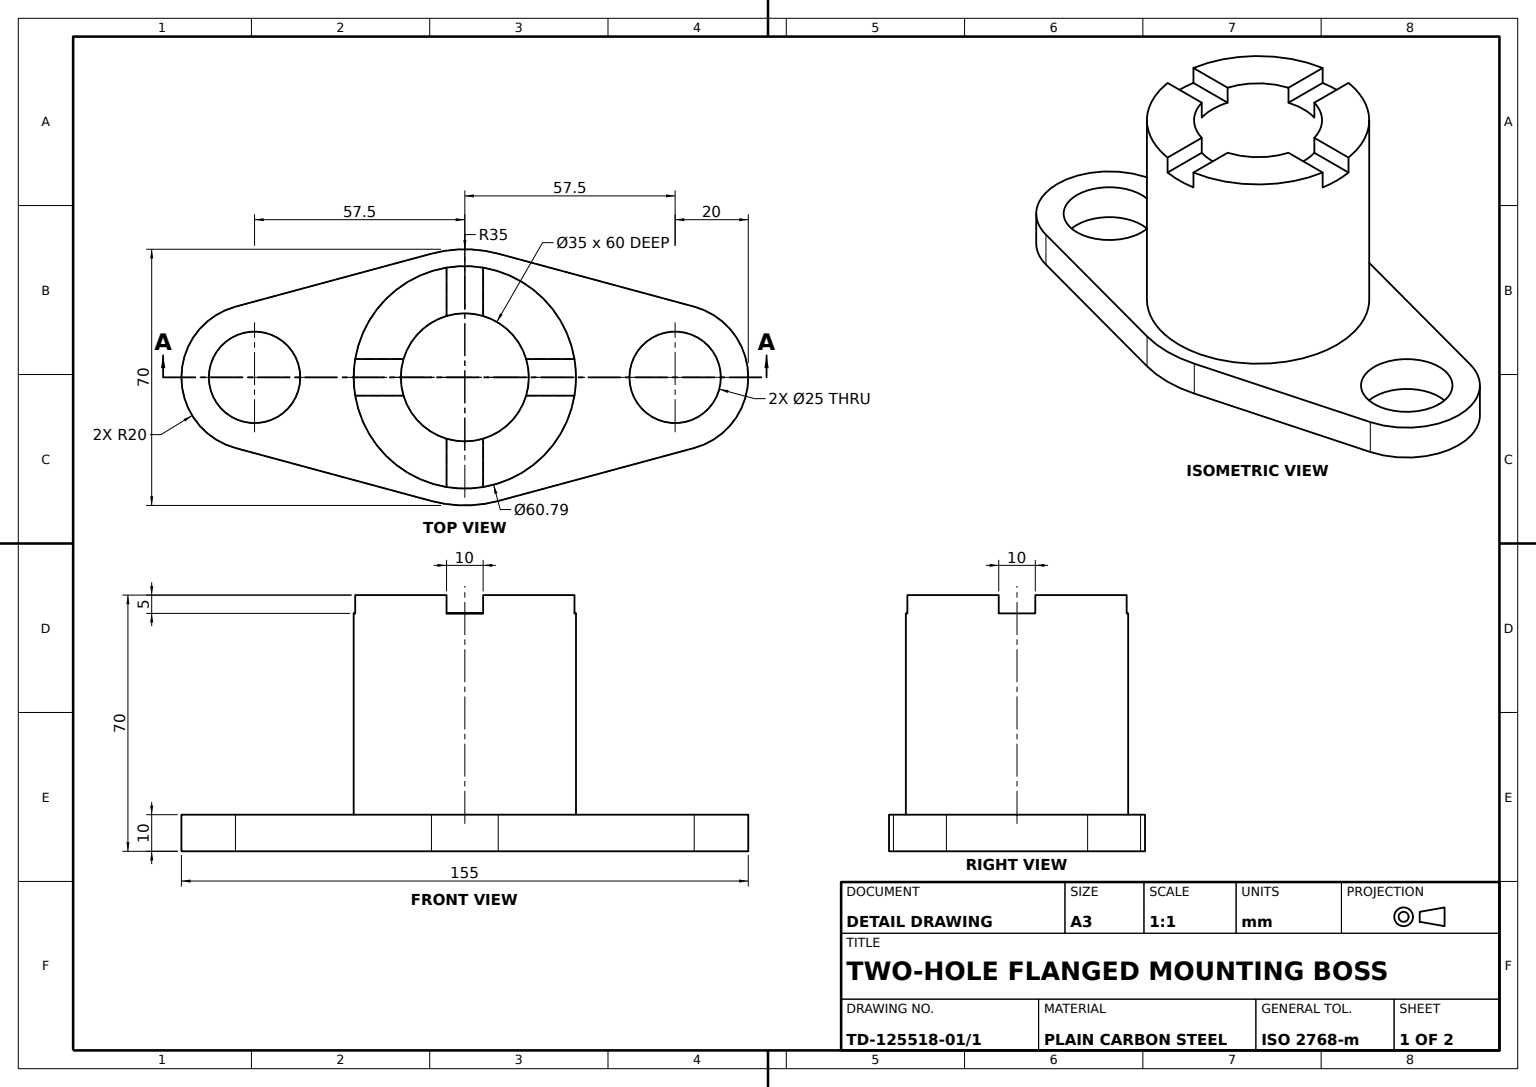
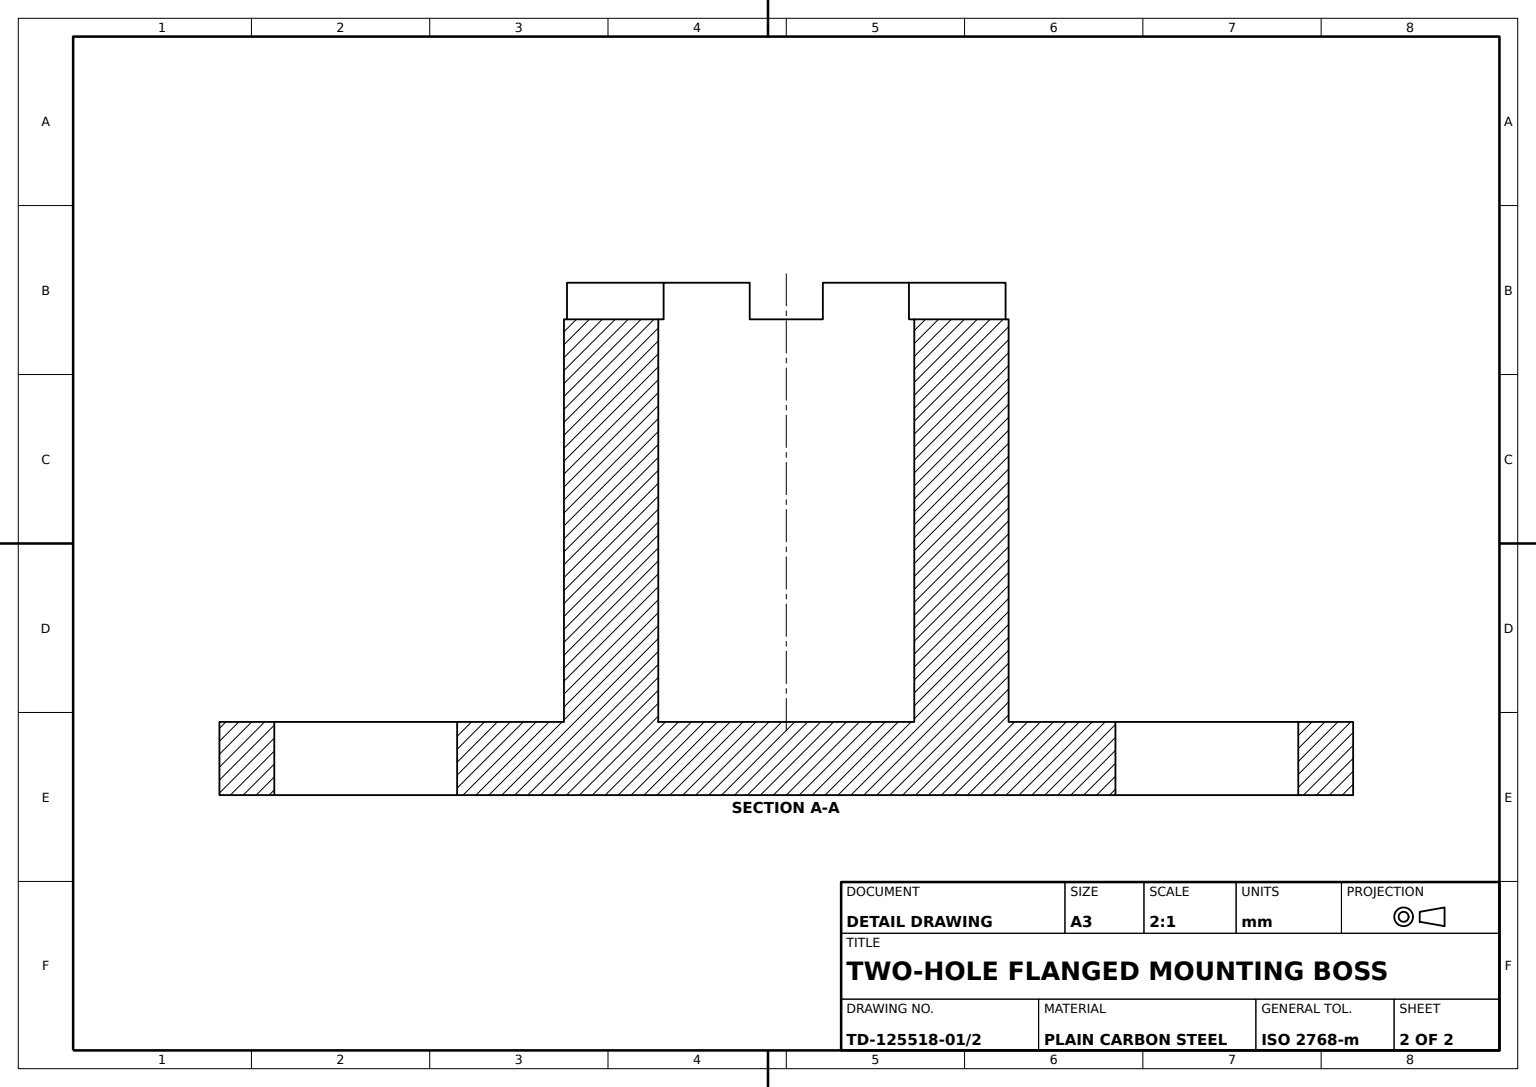
SolidWorks part; units mm, degrees
material "Plain Carbon Steel"
ref_plane "Front Plane" through (0, 0, 0) normal (0, 0, 1) x (1, 0, 0)
ref_plane "Top Plane" through (0, 0, 0) normal (0, 1, 0) x (1, 0, 0)
ref_plane "Right Plane" through (0, 0, 0) normal (1, 0, 0) x (0, 0, -1)
sketch "Base Plate Profile" plane through (0, 0, 0) normal (0, 1, 0) x (1, 0, 0)
  line L0 (0, -57.5) -> (0, 57.5) construction
  line L1 (-133.8812, 0) -> (133.8812, 0) construction
  line L2 (19.3075, -62.7174) -> (33.7881, -9.1304)
  line L3 (19.3075, 62.7174) -> (33.7881, 9.1304)
  line L4 (-19.3075, -62.7174) -> (-33.7881, -9.1304)
  line L5 (-19.3075, 62.7174) -> (-33.7881, 9.1304)
  arc A0 (-33.7881, 9.1304) -> (-33.7881, -9.1304) centre (0, 0) ccw
  arc A3 (-19.3075, -62.7174) -> (19.3075, -62.7174) centre (0, -57.5) ccw
  arc A4 (19.3075, 62.7174) -> (-19.3075, 62.7174) centre (0, 57.5) ccw
  arc A5 (33.7881, -9.1304) -> (33.7881, 9.1304) centre (0, 0) ccw
  point P4 (0, 0)
  point P8 (0, 0)
  dimension "D1" = 70
  dimension "D2" = 40
  dimension "D3" = 40
  dimension "D4" = 57.5
extrude "Base Plate" add sketch "Base Plate Profile" along normal blind 10
sketch "Mounting Holes Profile" plane through (0, 10, 0) normal (0, 1, 0) x (1, 0, 0)
  circle A0 centre (0, 57.5) radius 12.5
  circle A1 centre (0, -57.5) radius 12.5
  dimension "D1" = 25
extrude "Mounting Holes 2x" cut sketch "Mounting Holes Profile" against normal through all both
sketch "Hub Profile" plane through (0, 10, 0) normal (0, 1, 0) x (1, 0, 0)
  circle A0 centre (0, 0) radius 30.3952
  dimension "D1" = 60.7903
extrude "Hub" add sketch "Hub Profile" along normal blind 60
sketch "Bore Profile Ø35" plane through (0, 70, 0) normal (0, 1, 0) x (1, 0, 0)
  circle A1 centre (0, 0) radius 17.5
  dimension "D1" = 35
extrude "Bore Ø35" cut sketch "Bore Profile Ø35" against normal up to surface (60 mm away) up to face at (0, 10, 30.3952)
sketch "Cross Slots Profile" plane through (0, 70, 0) normal (0, 1, 0) x (1, 0, 0)
  line L0 (-16.7705, -5) -> (-29.9811, -5)
  line L1 (-5, -16.7705) -> (-5, -29.9811)
  line L2 (5, -16.7705) -> (5, -29.9811)
  line L3 (-16.7705, 5) -> (-29.9811, 5)
  line L4 (-5, 16.7705) -> (-5, 29.9811)
  line L5 (5, 16.7705) -> (5, 29.9811)
  line L6 (16.7705, 5) -> (29.9811, 5)
  line L7 (16.7705, -5) -> (29.9811, -5)
  arc A0 (-5, -16.7705) -> (5, -16.7705) centre (0, 0) ccw
  arc A1 (-5, -29.9811) -> (5, -29.9811) centre (0, 0) ccw
  arc A2 (-16.7705, 5) -> (-16.7705, -5) centre (0, 0) ccw
  arc A3 (-29.9811, 5) -> (-29.9811, -5) centre (0, 0) ccw
  arc A4 (5, 16.7705) -> (-5, 16.7705) centre (0, 0) ccw
  arc A5 (5, 29.9811) -> (-5, 29.9811) centre (0, 0) ccw
  arc A6 (16.7705, -5) -> (16.7705, 5) centre (0, 0) ccw
  arc A7 (29.9811, -5) -> (29.9811, 5) centre (0, 0) ccw
  circle A8 centre (0, 0) radius 17.5 construction
  point P21 (0, 0)
  dimension "D3" = 30.3952
  dimension "D2" = 17.5
  dimension "D4" = 5
  dimension "D1" = 4
extrude "Cross Slots 4x" cut sketch "Cross Slots Profile" against normal blind 5
